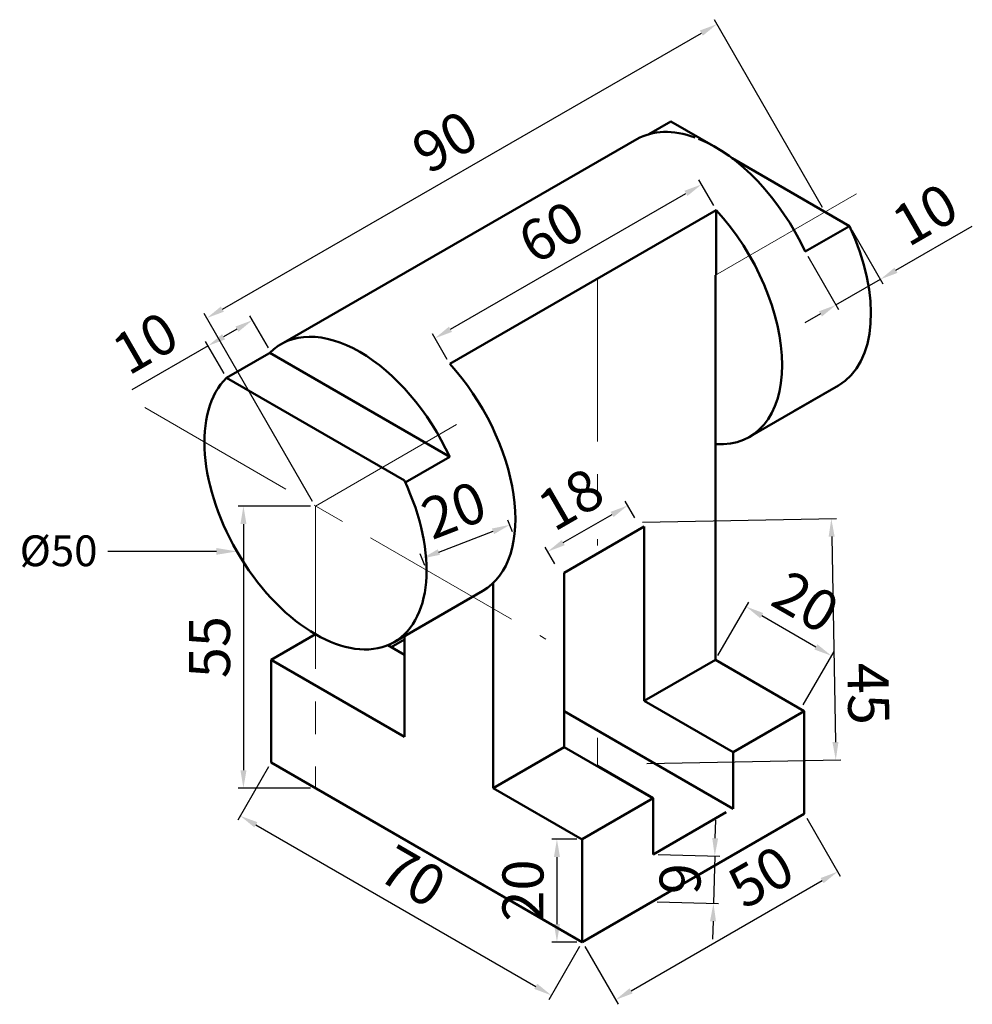
# Model space of a CAD drawing. Units: millimetres. Extents: x 2493 to 2679, y 1649 to 1841.
import ezdxf
from ezdxf import colors
from ezdxf.entities.mleader import LeaderData, LeaderLine
from ezdxf.math import Vec2, Vec3

# ---------------------------------------------------------------- set-up
doc = ezdxf.new("R2010")
doc.units = ezdxf.units.MM
doc.linetypes.add('CENTER', pattern=[50.8, 31.75, -6.35, 6.35, -6.35])
for name, color, linetype, lineweight in [('M-CNTR', 1, 'CENTER', 18), ('M-DIMS', 3, 'Continuous', 25), ('M-OUTL', 7, 'Continuous', 50), ('M-TEXT', 3, 'Continuous', 25)]:
    doc.layers.add(name, color=color, linetype=linetype, lineweight=lineweight)
doc.styles.get("Standard").update_dxf_attribs({"font": 'arial.ttf'})
doc.dimstyles.new('AM_ISO$0', dxfattribs={"dimtxt": 8, "dimasz": 3.5, "dimexe": 1, "dimexo": 1, "dimgap": 1.5, "dimtad": 1, "dimdsep": 46, "dimtxsty": 'Standard', "dimcen": 0, "dimclrd": 256, "dimclre": 256, "dimclrt": 2, "dimadec": 0, "dimazin": 2, "dimtp": 0.1, "dimtm": 0.1, "dimtfac": 0.71, "dimtmove": 0, "dimatfit": 3, "dimfxl": 1, "dimlwd": -1, "dimlwe": -1, "dimarcsym": 1})

# ---------------------------------------------------------------- blocks, each defined once
blk = doc.blocks.new('*D3')
at = {"layer": 'Defpoints', "color": 0, "transparency": 16777216}
for p in [(2611.48, 1746.23), (2613.37, 1742.96), (2597.78, 1733.96)]:
    blk.add_point(p, dxfattribs=at)
at = {"layer": 'M-DIMS', "color": 0, "linetype": 'ByBlock', "transparency": 16777216}
for p, q in [((2612.87, 1743.82), (2610.98, 1747.1)), ((2598.92, 1738.98), (2608.45, 1744.48)), ((2597.28, 1734.82), (2595.39, 1738.1))]:
    blk.add_line(p, q, dxfattribs=at)
at = {"layer": 'M-DIMS', "color": 0, "transparency": 16777216}
for points in [[(2608.16, 1744.99), (2608.74, 1743.98), (2611.48, 1746.23)], [(2598.63, 1739.49), (2599.22, 1738.48), (2595.89, 1737.23)]]:
    blk.add_solid(points, dxfattribs=at)
at = {"layer": 'M-DIMS', "color": 0, "transparency": 16777216, "insert": (2600.89, 1746.57), "char_height": 8, "attachment_point": 5, "rotation": 30}
blk.add_mtext('18', dxfattribs=at)
blk = doc.blocks.new('*D4')
at = {"layer": 'Defpoints', "color": 0, "transparency": 16777216}
for p in [(2616.45, 1678.18), (2616.21, 1668.97), (2628.2, 1668.66)]:
    blk.add_point(p, dxfattribs=at)
at = {"layer": 'M-DIMS', "color": 0, "linetype": 'ByBlock', "transparency": 16777216}
for p, q in [((2628.54, 1681.36), (2628.63, 1684.86)), ((2617.45, 1678.15), (2629.45, 1677.84)), ((2628.45, 1677.86), (2628.2, 1668.66)), ((2617.21, 1668.95), (2629.2, 1668.63)), ((2628.11, 1665.16), (2628.02, 1661.66))]:
    blk.add_line(p, q, dxfattribs=at)
at = {"layer": 'M-DIMS', "color": 0, "transparency": 16777216}
for points in [[(2627.96, 1681.38), (2629.12, 1681.35), (2628.45, 1677.86)], [(2627.53, 1665.17), (2628.7, 1665.14), (2628.2, 1668.66)]]:
    blk.add_solid(points, dxfattribs=at)
at = {"layer": 'M-DIMS', "color": 0, "transparency": 16777216, "insert": (2622.74, 1673.41), "char_height": 8, "attachment_point": 5, "rotation": 88.488}
blk.add_mtext('9', dxfattribs=at)
blk = doc.blocks.new('*D5')
at = {"layer": 'Defpoints', "color": 0, "transparency": 16777216}
for p in [(2602.6, 1681.18), (2597.69, 1661.11), (2602.6, 1661.11)]:
    blk.add_point(p, dxfattribs=at)
at = {"layer": 'M-DIMS', "color": 0, "linetype": 'ByBlock', "transparency": 16777216}
for p, q in [((2601.6, 1681.18), (2596.69, 1681.18)), ((2597.69, 1677.68), (2597.69, 1664.61)), ((2601.6, 1661.11), (2596.69, 1661.11))]:
    blk.add_line(p, q, dxfattribs=at)
at = {"layer": 'M-DIMS', "color": 0, "transparency": 16777216}
for points in [[(2597.11, 1677.68), (2598.28, 1677.68), (2597.69, 1681.18)], [(2597.11, 1664.61), (2598.28, 1664.61), (2597.69, 1661.11)]]:
    blk.add_solid(points, dxfattribs=at)
at = {"layer": 'M-DIMS', "color": 0, "transparency": 16777216, "insert": (2592.11, 1671.15), "char_height": 8, "attachment_point": 5, "rotation": 90}
blk.add_mtext('20', dxfattribs=at)
blk = doc.blocks.new('*D6')
at = {"layer": 'Defpoints', "color": 0, "transparency": 16777216}
for p in [(2541.97, 1696.11), (2602.6, 1661.11), (2596.6, 1650.72)]:
    blk.add_point(p, dxfattribs=at)
at = {"layer": 'M-DIMS', "color": 0, "linetype": 'ByBlock', "transparency": 16777216}
for p, q in [((2541.47, 1695.25), (2535.47, 1684.86)), ((2539, 1683.97), (2593.56, 1652.47)), ((2602.1, 1660.25), (2596.1, 1649.86))]:
    blk.add_line(p, q, dxfattribs=at)
at = {"layer": 'M-DIMS', "color": 0, "transparency": 16777216}
for points in [[(2539.3, 1684.48), (2538.71, 1683.47), (2535.97, 1685.72)], [(2593.86, 1652.98), (2593.27, 1651.97), (2596.6, 1650.72)]]:
    blk.add_solid(points, dxfattribs=at)
at = {"layer": 'M-DIMS', "color": 0, "transparency": 16777216, "insert": (2569.08, 1673.06), "char_height": 8, "attachment_point": 5, "rotation": 330}
blk.add_mtext('70', dxfattribs=at)
blk = doc.blocks.new('*D7')
at = {"layer": 'Defpoints', "color": 0, "transparency": 16777216}
for p in [(2529.7, 1777.37), (2541.97, 1776.11), (2533.31, 1771.11)]:
    blk.add_point(p, dxfattribs=at)
at = {"layer": 'M-DIMS', "color": 0, "linetype": 'ByBlock', "transparency": 16777216}
for p, q in [((2541.47, 1776.98), (2537.86, 1783.23)), ((2535.33, 1780.62), (2532.73, 1779.12)), ((2532.81, 1771.98), (2529.2, 1778.23)), ((2529.7, 1777.37), (2514.83, 1768.78))]:
    blk.add_line(p, q, dxfattribs=at)
at = {"layer": 'M-DIMS', "color": 0, "transparency": 16777216}
for points in [[(2535.04, 1781.12), (2535.62, 1780.11), (2538.36, 1782.37)], [(2532.44, 1779.62), (2533.03, 1778.61), (2529.7, 1777.37)]]:
    blk.add_solid(points, dxfattribs=at)
at = {"layer": 'M-DIMS', "color": 0, "transparency": 16777216, "insert": (2517.96, 1777.03), "char_height": 8, "attachment_point": 5, "rotation": 30}
blk.add_mtext('10', dxfattribs=at)
blk = doc.blocks.new('*D8')
at = {"layer": 'Defpoints', "color": 0, "transparency": 16777216}
for p in [(2645.9, 1686.11), (2652.41, 1674.83), (2602.6, 1661.11)]:
    blk.add_point(p, dxfattribs=at)
at = {"layer": 'M-DIMS', "color": 0, "linetype": 'ByBlock', "transparency": 16777216}
for p, q in [((2646.4, 1685.25), (2652.91, 1673.97)), ((2612.14, 1651.58), (2649.38, 1673.08)), ((2603.1, 1660.25), (2609.61, 1648.97))]:
    blk.add_line(p, q, dxfattribs=at)
at = {"layer": 'M-DIMS', "color": 0, "transparency": 16777216}
for points in [[(2649.09, 1673.59), (2649.67, 1672.58), (2652.41, 1674.83)], [(2611.85, 1652.09), (2612.43, 1651.08), (2609.11, 1649.83)]]:
    blk.add_solid(points, dxfattribs=at)
at = {"layer": 'M-DIMS', "color": 0, "transparency": 16777216, "insert": (2637.96, 1672.94), "char_height": 8, "attachment_point": 5, "rotation": 30}
blk.add_mtext('50', dxfattribs=at)
blk = doc.blocks.new('*D9')
at = {"layer": 'Defpoints', "color": 0, "transparency": 16777216}
for p in [(2613.37, 1742.96), (2614.24, 1695.9), (2652.04, 1696.6)]:
    blk.add_point(p, dxfattribs=at)
at = {"layer": 'M-DIMS', "color": 0, "linetype": 'ByBlock', "transparency": 16777216}
for p, q in [((2614.37, 1742.98), (2652.17, 1743.67)), ((2651.24, 1740.15), (2651.97, 1700.1)), ((2615.24, 1695.92), (2653.04, 1696.62))]:
    blk.add_line(p, q, dxfattribs=at)
at = {"layer": 'M-DIMS', "color": 0, "transparency": 16777216}
for points in [[(2651.82, 1740.17), (2650.65, 1740.14), (2651.17, 1743.65)], [(2652.56, 1700.11), (2651.39, 1700.09), (2652.04, 1696.6)]]:
    blk.add_solid(points, dxfattribs=at)
at = {"layer": 'M-DIMS', "color": 0, "transparency": 16777216, "insert": (2657.37, 1709.5), "char_height": 8, "attachment_point": 5, "rotation": 271.0543}
blk.add_mtext('45', dxfattribs=at)
blk = doc.blocks.new('*D10')
at = {"layer": 'Defpoints', "color": 0, "transparency": 16777216}
for p in [(2628.87, 1840.08), (2649.98, 1803.47), (2550.56, 1746.16)]:
    blk.add_point(p, dxfattribs=at)
at = {"layer": 'M-DIMS', "color": 0, "linetype": 'ByBlock', "transparency": 16777216}
for p, q in [((2649.48, 1804.34), (2628.37, 1840.95)), ((2532.48, 1784.52), (2625.84, 1838.34)), ((2550.06, 1747.02), (2528.95, 1783.64))]:
    blk.add_line(p, q, dxfattribs=at)
at = {"layer": 'M-DIMS', "color": 0, "transparency": 16777216}
for points in [[(2625.55, 1838.84), (2626.13, 1837.83), (2628.87, 1840.08)], [(2532.19, 1785.02), (2532.77, 1784.01), (2529.45, 1782.77)]]:
    blk.add_solid(points, dxfattribs=at)
at = {"layer": 'M-DIMS', "color": 0, "transparency": 16777216, "insert": (2576.38, 1816.27), "char_height": 8, "attachment_point": 5, "rotation": 29.9619}
blk.add_mtext('90', dxfattribs=at)
blk = doc.blocks.new('*D11')
at = {"layer": 'Defpoints', "color": 0, "transparency": 16777216}
for p in [(2651.2, 1716.91), (2628.58, 1716.11), (2645.2, 1706.51)]:
    blk.add_point(p, dxfattribs=at)
at = {"layer": 'M-DIMS', "color": 0, "linetype": 'ByBlock', "transparency": 16777216}
for p, q in [((2629.08, 1716.98), (2635.08, 1727.37)), ((2637.61, 1724.76), (2648.17, 1718.66)), ((2645.7, 1707.38), (2651.7, 1717.77))]:
    blk.add_line(p, q, dxfattribs=at)
at = {"layer": 'M-DIMS', "color": 0, "transparency": 16777216}
for points in [[(2637.9, 1725.26), (2637.32, 1724.25), (2634.58, 1726.51)], [(2648.46, 1719.16), (2647.88, 1718.15), (2651.2, 1716.91)]]:
    blk.add_solid(points, dxfattribs=at)
at = {"layer": 'M-DIMS', "color": 0, "transparency": 16777216, "insert": (2645.68, 1726.54), "char_height": 8, "attachment_point": 5, "rotation": 330}
blk.add_mtext('20', dxfattribs=at)
blk = doc.blocks.new('*D12')
at = {"layer": 'Defpoints', "color": 0, "transparency": 16777216}
for p in [(2588.51, 1742.45), (2589.38, 1740.16), (2572.28, 1733.61)]:
    blk.add_point(p, dxfattribs=at)
at = {"layer": 'M-DIMS', "color": 0, "linetype": 'ByBlock', "transparency": 16777216}
for p, q in [((2589.02, 1741.1), (2588.15, 1743.38)), ((2574.68, 1737.15), (2585.24, 1741.19)), ((2571.93, 1734.55), (2571.05, 1736.83))]:
    blk.add_line(p, q, dxfattribs=at)
at = {"layer": 'M-DIMS', "color": 0, "transparency": 16777216}
for points in [[(2585.03, 1741.74), (2585.45, 1740.65), (2588.51, 1742.45)], [(2574.47, 1737.69), (2574.89, 1736.6), (2571.41, 1735.9)]]:
    blk.add_solid(points, dxfattribs=at)
at = {"layer": 'M-DIMS', "color": 0, "transparency": 16777216, "insert": (2577.96, 1744.39), "char_height": 8, "attachment_point": 5, "rotation": 20.9572}
blk.add_mtext('20', dxfattribs=at)
blk = doc.blocks.new('*D13')
at = {"layer": 'Defpoints', "color": 0, "transparency": 16777216}
for p in [(2654.74, 1800.72), (2646.08, 1795.72), (2660.74, 1790.33)]:
    blk.add_point(p, dxfattribs=at)
at = {"layer": 'M-DIMS', "color": 0, "linetype": 'ByBlock', "transparency": 16777216}
for p, q in [((2655.24, 1799.86), (2661.24, 1789.47)), ((2663.77, 1792.08), (2678.65, 1800.67)), ((2646.58, 1794.86), (2652.58, 1784.47)), ((2652.08, 1785.33), (2660.74, 1790.33)), ((2649.05, 1783.58), (2646.02, 1781.83))]:
    blk.add_line(p, q, dxfattribs=at)
at = {"layer": 'M-DIMS', "color": 0, "transparency": 16777216}
for points in [[(2663.48, 1792.59), (2664.06, 1791.58), (2660.74, 1790.33)], [(2648.76, 1784.09), (2649.34, 1783.08), (2652.08, 1785.33)]]:
    blk.add_solid(points, dxfattribs=at)
at = {"layer": 'M-DIMS', "color": 0, "transparency": 16777216, "insert": (2669.93, 1802.09), "char_height": 8, "attachment_point": 5, "rotation": 30}
blk.add_mtext('10', dxfattribs=at)
blk = doc.blocks.new('*D14')
at = {"layer": 'Defpoints', "color": 0, "transparency": 16777216}
for p in [(2625.87, 1808.83), (2628.75, 1803.84), (2576.79, 1773.84)]:
    blk.add_point(p, dxfattribs=at)
at = {"layer": 'M-DIMS', "color": 0, "linetype": 'ByBlock', "transparency": 16777216}
for p, q in [((2628.25, 1804.7), (2625.37, 1809.7)), ((2576.94, 1780.58), (2622.84, 1807.08)), ((2576.29, 1774.7), (2573.41, 1779.7))]:
    blk.add_line(p, q, dxfattribs=at)
at = {"layer": 'M-DIMS', "color": 0, "transparency": 16777216}
for points in [[(2622.54, 1807.59), (2623.13, 1806.58), (2625.87, 1808.83)], [(2576.64, 1781.09), (2577.23, 1780.08), (2573.91, 1778.83)]]:
    blk.add_solid(points, dxfattribs=at)
at = {"layer": 'M-DIMS', "color": 0, "transparency": 16777216, "insert": (2597.09, 1798.67), "char_height": 8, "attachment_point": 5, "rotation": 30}
blk.add_mtext('60', dxfattribs=at)
blk = doc.blocks.new('*D15')
at = {"layer": 'Defpoints', "color": 0, "transparency": 16777216}
for p in [(2550.63, 1746.11), (2536.59, 1691.11), (2550.63, 1691.11)]:
    blk.add_point(p, dxfattribs=at)
at = {"layer": 'M-DIMS', "linetype": 'ByBlock', "transparency": 16777216}
for p, q in [((2549.63, 1746.11), (2535.59, 1746.11)), ((2536.59, 1742.61), (2536.59, 1694.61)), ((2549.63, 1691.11), (2535.59, 1691.11))]:
    blk.add_line(p, q, dxfattribs=at)
at = {"layer": 'M-DIMS', "transparency": 16777216}
for points in [[(2536.01, 1742.61), (2537.18, 1742.61), (2536.59, 1746.11)], [(2536.01, 1694.61), (2537.18, 1694.61), (2536.59, 1691.11)]]:
    blk.add_solid(points, dxfattribs=at)
at = {"layer": 'M-DIMS', "color": 2, "transparency": 16777216, "insert": (2531.02, 1718.61), "char_height": 8, "attachment_point": 5, "rotation": 90}
blk.add_mtext('55', dxfattribs=at)

msp = doc.modelspace()

# ---------------------------------------------------------------- linework, layer by layer
at = {"layer": 'M-CNTR'}
for p, q in [((2628.576, 1791.113), (2660.126, 1809.329)), ((2605.577, 1790.456), (2605.577, 1738.458)), ((2517.373, 1765.317), (2595.528, 1720.194)), ((2550.634, 1746.113), (2583.263, 1764.952)), ((2550.634, 1746.113), (2550.634, 1691.113)), ((2605.577, 1700.901), (2605.577, 1695.458))]:
    msp.add_line(p, q, dxfattribs=at)
at = {"layer": 'M-OUTL'}
for p, q in [((2615.585, 1818.613), (2619.916, 1821.113)), ((2628.576, 1816.113), (2619.916, 1821.113)), ((2543.946, 1777.696), (2613.275, 1817.635)), ((2654.738, 1800.724), (2631.862, 1813.926)), ((2576.79, 1773.835), (2628.751, 1803.835)), ((2628.751, 1803.835), (2628.751, 1791.215)), ((2646.078, 1795.724), (2654.738, 1800.724)), ((2628.576, 1716.113), (2628.576, 1791.113)), ((2533.313, 1771.113), (2541.973, 1776.113)), ((2541.721, 1775.968), (2576.79, 1755.721)), ((2567.954, 1751.113), (2533.313, 1771.113)), ((2635.225, 1759.597), (2652.545, 1769.597)), ((2643.885, 1764.597), (2652.545, 1769.597)), ((2550.634, 1761.113), (2567.954, 1751.113)), ((2576.79, 1755.721), (2568.136, 1750.724)), ((2568.136, 1750.724), (2576.79, 1755.721)), ((2599.131, 1733.113), (2614.719, 1742.113)), ((2614.719, 1708.113), (2614.719, 1742.113)), ((2599.131, 1699.113), (2599.131, 1733.113)), ((2585.275, 1691.113), (2585.275, 1731.113)), ((2583.263, 1729.597), (2565.943, 1719.597)), ((2565.943, 1719.597), (2583.263, 1729.597)), ((2541.973, 1716.113), (2550.634, 1721.113)), ((2567.954, 1701.113), (2567.954, 1720.758)), ((2567.954, 1717.113), (2564.705, 1718.989)), ((2565.356, 1718.613), (2567.954, 1720.113)), ((2541.973, 1696.113), (2541.973, 1716.113)), ((2567.954, 1701.113), (2541.973, 1716.113)), ((2614.719, 1708.113), (2628.576, 1716.113)), ((2645.896, 1706.113), (2628.576, 1716.113)), ((2632.04, 1698.113), (2614.719, 1708.113)), ((2599.131, 1706.113), (2632.04, 1687.113)), ((2632.04, 1698.113), (2645.896, 1706.113)), ((2645.896, 1686.113), (2645.896, 1706.113)), ((2585.275, 1691.113), (2599.131, 1699.113)), ((2616.451, 1689.113), (2599.131, 1699.113)), ((2632.04, 1687.113), (2632.04, 1698.113)), ((2602.595, 1661.113), (2541.973, 1696.113)), ((2616.452, 1689.18), (2605.577, 1695.458)), ((2550.634, 1691.113), (2572.284, 1678.613)), ((2602.595, 1681.113), (2585.275, 1691.113)), ((2602.595, 1681.18), (2616.452, 1689.18)), ((2616.452, 1689.18), (2616.452, 1678.18)), ((2602.595, 1661.113), (2645.896, 1686.113)), ((2616.452, 1678.18), (2630.692, 1686.401)), ((2602.595, 1661.113), (2602.595, 1681.18)), ((2572.284, 1678.613), (2602.595, 1661.113))]:
    msp.add_line(p, q, dxfattribs=at)
for centre, start_param, end_param in [((2628.576, 1791.113), 2.5403284, 3.141042), ((2628.576, 1791.113), 7.6979566, 8.7921912), ((2619.916, 1786.113), 5.9181651, 8.2190018), ((2637.236, 1796.113), 6.2831853, 7.6979566), ((2559.255, 1751.179), 7.6954336, 9.583326), ((2567.954, 1756.113), 6.2831853, 8.2190018), ((2550.634, 1746.113), 3.2834897, 7.7120846)]:
    msp.add_ellipse(centre, major_axis=(15.309, -26.517), ratio=0.5773503, start_param=start_param, end_param=end_param, dxfattribs=at)

# ---------------------------------------------------------------- dimensions: what is measured, and where the dimension line sits
at = {"layer": 'M-DIMS'}
for base, p1, p2, angle, text, picture, middle in [((2628.873, 1840.084), (2550.557, 1746.157), (2649.98, 1803.471), 29.96191, '90', '*D10', (2579.173, 1811.434)), ((2652.039, 1696.597), (2613.371, 1742.958), (2614.237, 1695.901), 271.05434, '45', '*D9', (2651.804, 1709.394))]:
    dim = msp.add_linear_dim(base=base, p1=p1, p2=p2, angle=angle, text=text, dimstyle='AM_ISO$0', override={"dimclrd": 0, "dimclre": 0, "dimclrt": 0}, dxfattribs=at)
    dim.commit()
    dim.dimension.update_dxf_attribs({"geometry": picture, "text_midpoint": middle, "dimtype": 161})
for p1, p2, distance, override, picture, middle in [((2576.79, 1773.835), (2628.751, 1803.835), 5.769, {"dimclrd": 0, "dimclre": 0, "dimclrt": 0}, '*D14', (2597.094, 1798.668)), ((2646.078, 1795.724), (2654.738, 1800.724), -12, {"dimpost": '', "dimclrd": 0, "dimclre": 0, "dimclrt": 0}, '*D13', (2669.932, 1802.088)), ((2541.973, 1776.113), (2533.313, 1771.113), -7.22, {"dimpost": '', "dimclrd": 0, "dimclre": 0, "dimclrt": 0}, '*D7', (2517.956, 1777.033)), ((2597.783, 1733.958), (2613.371, 1742.958), 3.78, {"dimpost": '', "dimclrd": 0, "dimclre": 0, "dimclrt": 0}, '*D3', (2600.895, 1746.568)), ((2541.973, 1696.113), (2602.595, 1661.113), -12, {"dimclrd": 0, "dimclre": 0, "dimclrt": 0}, '*D6', (2569.077, 1673.057))]:
    dim = msp.add_aligned_dim(p1=p1, p2=p2, distance=distance, dimstyle='AM_ISO$0', override=override, dxfattribs=at)
    dim.commit()
    dim.dimension.update_dxf_attribs({"geometry": picture, "text_midpoint": middle})
for p1, p2, distance, text, picture, middle in [((2572.284, 1733.613), (2589.382, 1740.162), 2.446, '20', '*D12', (2577.96, 1744.387)), ((2628.576, 1716.113), (2645.202, 1706.514), 12, '20', '*D11', (2645.681, 1726.542)), ((2616.452, 1678.18), (2616.209, 1668.973), 12, '9', '*D4', (2622.743, 1673.407)), ((2602.595, 1681.18), (2602.595, 1661.113), -4.901, '20', '*D5', (2592.109, 1671.147))]:
    dim = msp.add_aligned_dim(p1=p1, p2=p2, distance=distance, text=text, dimstyle='AM_ISO$0', override={"dimpost": '', "dimclrd": 0, "dimclre": 0, "dimclrt": 0}, dxfattribs=at)
    dim.commit()
    dim.dimension.update_dxf_attribs({"geometry": picture, "text_midpoint": middle})
dim = msp.add_linear_dim(base=(2536.593, 1691.113), p1=(2550.634, 1746.113), p2=(2550.634, 1691.113), angle=270, dimstyle='AM_ISO$0', override={"dimrnd": 0}, dxfattribs=at)
dim.commit()
dim.dimension.update_dxf_attribs({"geometry": '*D15', "text_midpoint": (2531.025, 1718.613)})
dim = msp.add_linear_dim(base=(2652.409, 1674.833), p1=(2602.595, 1661.113), p2=(2645.896, 1686.113), angle=30, dimstyle='AM_ISO$0', override={"dimclrd": 0, "dimclre": 0, "dimclrt": 0}, dxfattribs=at)
dim.commit()
dim.dimension.update_dxf_attribs({"geometry": '*D8', "text_midpoint": (2640.752, 1668.103), "dimtype": 161})

# ---------------------------------------------------------------- leaders
at = {"layer": 'M-TEXT'}
ml = msp.add_multileader_mtext('Standard', dxfattribs=at)
ml.set_content('{\\C2;%%C50}', color=256)
ml.set_leader_properties()
ml.build(insert=Vec2(0, 0))
ctx = ml.context
ctx.base_point, ctx.char_height, ctx.plane_origin = Vec3(2491.042, 1737.275), 6, Vec3(2535.324, 1737.275)
ctx.text_align_type = 2
notes = []
notes.append((ctx, [(0, (1, 1, 0), (2518.145, 1737.275), (-1, 0), 8, [(0, [(2535.324, 1737.275)], 0, [])])]))
ctx.mtext.insert, ctx.mtext.alignment, ctx.mtext.flow_direction = Vec3(2508.145, 1740.395), 3, 5
for ctx, leaders in notes:
    for number, flags, end, landing, length, lines in leaders:
        leader = LeaderData()
        leader.index, (leader.has_last_leader_line, leader.has_dogleg_vector, leader.attachment_direction) = number, flags
        leader.last_leader_point, leader.dogleg_vector, leader.dogleg_length = Vec3(end), Vec3(landing), length
        for number, points, colour, breaks in lines:
            line = LeaderLine()
            line.index, line.vertices, line.color, line.breaks = number, Vec3.list(points), colors.encode_raw_color(colour), breaks
            leader.lines.append(line)
        ctx.leaders.append(leader)

doc.saveas('drawing.dxf')
